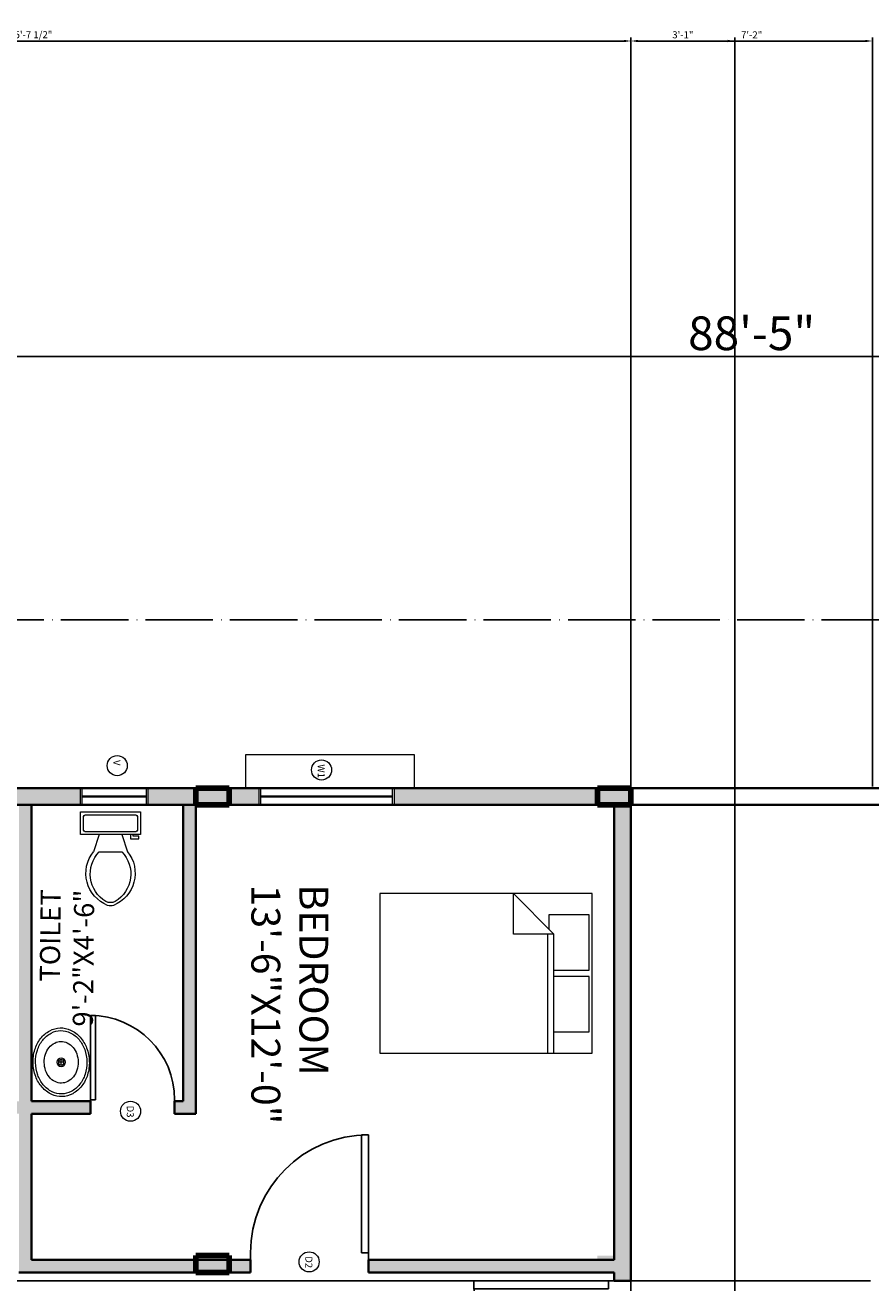
# Model space of a CAD drawing. Units: inches. Extents: x 7028582 to 7030319, y 63109697 to 63111305.
# Tile 12 of 18: x 7029446 to 7029748, y 63110857 to 63111305. Entities that reach past the tile are written whole.
import ezdxf

# ---------------------------------------------------------------- set-up
doc = ezdxf.new("R2010")
doc.units = ezdxf.units.IN
doc.linetypes.add('ACAD_ISO04W100', pattern=[30, 24, -3, 0, -3])
for name, color, linetype, lineweight in [('A-AREA-IDEN', 7, 'Continuous', 18), ('A-DOOR-IDEN', 20, 'Continuous', 13), ('A-FLOR-FIXT', 9, 'Continuous', 18), ('A-GLAZ-IDEN', 20, 'Continuous', 13), ('A-WALL-PATT', 8, 'Continuous', 13), ('C-ANNO-DIMS', 7, 'Continuous', 18), ('C-PROP', 1, 'ACAD_ISO04W100', 25), ('doors', 20, 'Continuous', 25), ('furniture', 9, 'Continuous', 18), ('PILLARS', 220, 'Continuous', 100), ('S-COLS-PATT', 220, 'Continuous', 100), ('walls', 6, 'Continuous', 35), ('WINDOW SHADOW', 9, 'Continuous', 13), ('windows', 5, 'Continuous', 18)]:
    doc.layers.add(name, color=color, linetype=linetype, lineweight=lineweight)
doc.styles.get("Standard").update_dxf_attribs({"font": 'arial.ttf'})
doc.dimstyles.new('ISO-25', dxfattribs={"dimtxt": 2.5, "dimasz": 2.5, "dimexe": 1.25, "dimexo": 0.625, "dimtad": 1, "dimlunit": 4, "dimtxsty": 'Standard', "dimcen": 2.5, "dimadec": 0, "dimazin": 0, "dimtfac": 1, "dimtmove": 0, "dimatfit": 3, "dimfxl": 1, "dimarcsym": 0})

# ---------------------------------------------------------------- blocks, each defined once
blk = doc.blocks.new('*U2')
for p, q in [((0, 0), (0, -5)), ((30, 0), (30, -5))]:
    blk.add_line(p, q)
blk.add_lwpolyline([(0, 0), (0, 30), (1.75, 30), (1.75, 0)], close=True)
blk.add_arc((0, 0), 30, 0, 90)
blk = doc.blocks.new('Toilet - top')
for p, q in [((9.5, -6), (9.5, -2)), ((-10, -8.5), (-8, -8.5)), ((-10, -9.5), (-10, -8.5)), ((-8, -8.5), (-8, -8)), ((-7, -8), (-7, -9.5)), ((-4, -8), (-6, -14)), ((4, -8), (6, -14)), ((-7, -9.5), (-10, -9.5)), ((4, -14), (-4, -14))]:
    blk.add_line(p, q)
blk.add_lwpolyline([(10.5, -8), (10.5, 0), (-10.5, 0), (-10.5, -8)], close=True)
for points in [[(-9.5, -2), (-9.5, -6)], [(8.5, -1), (-8.5, -1)], [(-8.5, -7), (8.5, -7)]]:
    blk.add_lwpolyline(points)
for centre, radius, start, end in [((-8.62, -1.88), 0.884, 81.8699, 188.1301), ((8.62, -1.88), 0.884, 351.8699, 98.1301), ((-8.62, -6.12), 0.884, 171.8699, 278.1301), ((8.62, -6.12), 0.884, 261.8699, 8.1301), ((3.52, -21.58), 12.17, 141.4691, 247.9714), ((4.2, -21.82), 11.33, 136.3677, 238.9468), ((-3.52, -21.58), 12.17, 292.0284, 38.5307), ((-4.2, -21.82), 11.33, 301.053, 43.6321), ((0, -27.88), 4, 245.7318, 294.2682), ((0, -29), 4, 254.8605, 285.1395)]:
    blk.add_arc(centre, radius, start, end)
blk = doc.blocks.new('Sink - Oval top')
for p, q in [((-1, 0), (1, 0)), ((0, 1), (0, -1))]:
    blk.add_line(p, q)
for points in [[(-12.23, 0.39, 0.117634), (-11.46, -3.36, 0.104469), (-8.88, -6.8, 0.090016), (-5.08, -9.07, 0.08192), (-0.32, -10.02, 0.08192), (4.49, -9.38, 0.090016), (8.42, -7.36, 0.104469), (11.22, -4.09, 0.117634), (12.23, -0.39, 0.117634), (11.46, 3.36, 0.104469), (8.88, 6.8, 0.090016), (5.08, 9.07, 0.08192), (0.32, 10.02, 0.08192), (-4.49, 9.38, 0.090016), (-8.42, 7.36, 0.104469), (-11.22, 4.09, 0.117634)], [(-11.29, 0.16, 0.118622), (-10.52, -3.25, 0.104678), (-8.07, -6.36, 0.089562), (-4.54, -8.37, 0.081185), (-0.13, -9.15, 0.081185), (4.3, -8.49, 0.089562), (7.89, -6.58, 0.104678), (10.42, -3.55, 0.118622), (11.29, -0.16, 0.118622), (10.52, 3.25, 0.104678), (8.07, 6.36, 0.089562), (4.54, 8.37, 0.081185), (0.13, 9.15, 0.081185), (-4.3, 8.49, 0.089562), (-7.89, 6.58, 0.104678), (-10.42, 3.55, 0.118622)], [(-7.42, 0.08, 0.118283), (-6.91, -2.17, 0.104607), (-5.29, -4.21, 0.089718), (-2.97, -5.53, 0.081436), (-0.07, -6.04, 0.081436), (2.84, -5.59, 0.089718), (5.2, -4.33, 0.104607), (6.86, -2.32, 0.118283), (7.42, -0.08, 0.118283), (6.91, 2.17, 0.104607), (5.29, 4.21, 0.089718), (2.97, 5.53, 0.081436), (0.07, 6.04, 0.081436), (-2.84, 5.59, 0.089718), (-5.2, 4.33, 0.104607), (-6.86, 2.32, 0.118283)]]:
    blk.add_lwpolyline(points, format="xyb", close=True)
for radius in [1.5, 1]:
    blk.add_circle((0, 0), radius)
blk = doc.blocks.new('Bed - Queen')
for p, q in [((0, -80.00003), (0, 0)), ((0, 0), (59.99999, 0)), ((59.99999, 0), (59.99999, -80.00003)), ((7.99999, -1.2), (28.79998, -1.2)), ((7.99999, -14.4), (7.99999, -1.2)), ((28.79998, -1.2), (28.79998, -14.4)), ((31.19999, -1.2), (51.99999, -1.2)), ((31.19999, -14.4), (31.19999, -1.2)), ((51.99999, -1.2), (51.99999, -16.4)), ((0, -14.4), (44.8, -14.4)), ((44.8, -16.8), (0, -16.8)), ((59.99999, -29.6), (44.8, -14.4)), ((44.8, -14.4), (44.8, -29.6)), ((51.99999, -16.4), (46.79936, -16.4)), ((44.8, -29.6), (59.99999, -29.6)), ((59.99999, -80.00003), (0, -80.00003))]:
    blk.add_line(p, q)
blk = doc.blocks.new('*D11')
at = {"layer": 'C-ANNO-DIMS', "color": 0, "lineweight": -2, "transparency": 16777216}
for p, q in [((7029174.71, 63111093.68), (7029174.71, 63111188.03)), ((7030233.21, 63111186.78), (7029177.21, 63111186.78)), ((7030235.71, 63111093.68), (7030235.71, 63111188.03))]:
    blk.add_line(p, q, dxfattribs=at)
at = {"layer": 'C-ANNO-DIMS', "color": 0, "lineweight": 100, "transparency": 16777216}
for points in [[(7029177.21, 63111187.2), (7029177.21, 63111186.36), (7029174.71, 63111186.78)], [(7030233.21, 63111187.2), (7030233.21, 63111186.36), (7030235.71, 63111186.78)]]:
    blk.add_solid(points, dxfattribs=at)
at = {"layer": 'Defpoints', "color": 0, "lineweight": 100, "transparency": 16777216}
for p in [(7029174.71, 63111186.78), (7029174.71, 63111093.06), (7030235.71, 63111093.06)]:
    blk.add_point(p, dxfattribs=at)
at = {"layer": 'C-ANNO-DIMS', "color": 0, "transparency": 16777216, "insert": (7029705.21, 63111193.53), "char_height": 12, "attachment_point": 5}
blk.add_mtext('88\'-5"', dxfattribs=at)
blk = doc.blocks.new('WIN-SASH-24')
for p, q in [((24.05, 6), (0, 6)), ((0.5, 6), (0.5, 0)), ((23.55, 0), (23.55, 6)), ((0, 0), (24.05, 0)), ((23.55, 3.2), (0.5, 3.2)), ((23.55, 2.8), (0.5, 2.8))]:
    blk.add_line(p, q)
blk = doc.blocks.new('WIN-SASH-48')
for p, q in [((48.05, 6), (0, 6)), ((0.5, 6), (0.5, 0)), ((47.55, 0), (47.55, 6)), ((47.55, 3.2), (0.5, 3.2)), ((47.55, 2.8), (0.5, 2.8)), ((0, 0), (48.05, 0))]:
    blk.add_line(p, q)
blk = doc.blocks.new('WINDOW-SHADE-HEAD-60')
for p, q in [((60.25, 11.9), (0, 11.9)), ((0, 11.9), (0, 0)), ((60.25, 0), (60.25, 11.9))]:
    blk.add_line(p, q)
blk = doc.blocks.new('COLUMN-RECT-PROFILE')
for p, q in [((11.91, 6), (0, 6)), ((0, 6), (0, 0)), ((11.91, 0), (11.91, 6)), ((0, 0), (11.91, 0))]:
    blk.add_line(p, q)
blk = doc.blocks.new('TAG-D2-MT-L')
blk.add_circle((3.58, 3.58), 3.58)
at = {"insert": (2.23, 5.6), "char_height": 2.5, "attachment_point": 7, "rotation": 270}
blk.add_mtext_dynamic_manual_height_columns('D2', width=2.5021, gutter_width=12.5, heights=[0], dxfattribs=at)
blk = doc.blocks.new('TAG-D3-MT-L')
blk.add_circle((3.58, 3.58), 3.58)
at = {"insert": (2.23, 5.6), "char_height": 2.5, "attachment_point": 7, "rotation": 270}
blk.add_mtext_dynamic_manual_height_columns('D3', width=2.5021, gutter_width=12.5, heights=[0], dxfattribs=at)
blk = doc.blocks.new('TAG-V-MT-L')
blk.add_circle((3.58, 3.58), 3.58)
at = {"insert": (2.23, 5.6), "char_height": 2.5, "attachment_point": 7, "rotation": 270}
blk.add_mtext_dynamic_manual_height_columns('V', width=2.5021, gutter_width=12.5, heights=[0], dxfattribs=at)
blk = doc.blocks.new('TAG-W1-MT-L')
blk.add_circle((3.58, 3.58), 3.58)
at = {"insert": (2.23, 5.6), "char_height": 2.5, "attachment_point": 7, "rotation": 270}
blk.add_mtext_dynamic_manual_height_columns('W1', width=2.5021, gutter_width=12.5, heights=[0], dxfattribs=at)
blk = doc.blocks.new('*D102')
at = {"layer": 'C-ANNO-DIMS', "color": 0, "lineweight": -2, "transparency": 16777216}
for p, q in [((7029662.21, 63111033.68), (7029662.21, 63111300.44)), ((7029664.71, 63111299.19), (7029745.71, 63111299.19)), ((7029748.21, 63111033.68), (7029748.21, 63111300.44))]:
    blk.add_line(p, q, dxfattribs=at)
at = {"layer": 'C-ANNO-DIMS', "color": 0, "lineweight": 100, "transparency": 16777216}
for points in [[(7029664.71, 63111299.61), (7029664.71, 63111298.77), (7029662.21, 63111299.19)], [(7029745.71, 63111299.61), (7029745.71, 63111298.77), (7029748.21, 63111299.19)]]:
    blk.add_solid(points, dxfattribs=at)
at = {"layer": 'Defpoints', "color": 0, "lineweight": 100, "transparency": 16777216}
for p in [(7029748.21, 63111299.19), (7029662.21, 63111033.06), (7029748.21, 63111033.06)]:
    blk.add_point(p, dxfattribs=at)
at = {"layer": 'C-ANNO-DIMS', "color": 0, "transparency": 16777216, "insert": (7029705.21, 63111301.07), "char_height": 2.5, "attachment_point": 5}
blk.add_mtext('7\'-2"', dxfattribs=at)
blk = doc.blocks.new('*D104')
at = {"layer": 'C-ANNO-DIMS', "color": 0, "lineweight": -2, "transparency": 16777216}
for p, q in [((7029747.58, 63110857.56), (7028586.23, 63110857.56)), ((7028587.48, 63110812.06), (7028587.48, 63110855.06)), ((7029747.58, 63110809.56), (7028586.23, 63110809.56))]:
    blk.add_line(p, q, dxfattribs=at)
at = {"layer": 'C-ANNO-DIMS', "color": 0, "lineweight": 100, "transparency": 16777216}
for points in [[(7028587.06, 63110855.06), (7028587.89, 63110855.06), (7028587.48, 63110857.56)], [(7028587.06, 63110812.06), (7028587.89, 63110812.06), (7028587.48, 63110809.56)]]:
    blk.add_solid(points, dxfattribs=at)
at = {"layer": 'Defpoints', "color": 0, "lineweight": 100, "transparency": 16777216}
for p in [(7028587.48, 63110857.56), (7029748.21, 63110857.56), (7029748.21, 63110809.56)]:
    blk.add_point(p, dxfattribs=at)
at = {"layer": 'C-ANNO-DIMS', "color": 0, "transparency": 16777216, "insert": (7028585.57, 63110833.56), "char_height": 2.5, "attachment_point": 5, "rotation": 90}
blk.add_mtext('4\'-0"', dxfattribs=at)
blk = doc.blocks.new('*D108')
at = {"layer": 'C-ANNO-DIMS', "color": 0, "lineweight": -2, "transparency": 16777216}
for p, q in [((7029662.21, 63110129.18), (7029662.21, 63111300.44)), ((7029664.71, 63111299.19), (7029696.71, 63111299.19)), ((7029699.21, 63110129.18), (7029699.21, 63111300.44))]:
    blk.add_line(p, q, dxfattribs=at)
at = {"layer": 'C-ANNO-DIMS', "color": 0, "lineweight": 100, "transparency": 16777216}
for points in [[(7029664.71, 63111299.61), (7029664.71, 63111298.77), (7029662.21, 63111299.19)], [(7029696.71, 63111299.61), (7029696.71, 63111298.77), (7029699.21, 63111299.19)]]:
    blk.add_solid(points, dxfattribs=at)
at = {"layer": 'Defpoints', "color": 0, "lineweight": 100, "transparency": 16777216}
for p in [(7029699.21, 63111299.19), (7029662.21, 63110128.56), (7029699.21, 63110128.56)]:
    blk.add_point(p, dxfattribs=at)
at = {"layer": 'C-ANNO-DIMS', "color": 0, "transparency": 16777216, "insert": (7029680.71, 63111301.09), "char_height": 2.5, "attachment_point": 5}
blk.add_mtext('3\'-1"', dxfattribs=at)
blk = doc.blocks.new('*D111')
at = {"layer": 'C-ANNO-DIMS', "color": 0, "lineweight": -2, "transparency": 16777216}
for p, q in [((7029234.71, 63111033.68), (7029234.71, 63111300.44)), ((7029237.21, 63111299.19), (7029659.71, 63111299.19)), ((7029662.21, 63111033.68), (7029662.21, 63111300.44))]:
    blk.add_line(p, q, dxfattribs=at)
at = {"layer": 'C-ANNO-DIMS', "color": 0, "lineweight": 100, "transparency": 16777216}
for points in [[(7029237.21, 63111299.61), (7029237.21, 63111298.77), (7029234.71, 63111299.19)], [(7029659.71, 63111299.61), (7029659.71, 63111298.77), (7029662.21, 63111299.19)]]:
    blk.add_solid(points, dxfattribs=at)
at = {"layer": 'Defpoints', "color": 0, "lineweight": 100, "transparency": 16777216}
for p in [(7029662.21, 63111299.19), (7029234.71, 63111033.06), (7029662.21, 63111033.06)]:
    blk.add_point(p, dxfattribs=at)
at = {"layer": 'C-ANNO-DIMS', "color": 0, "transparency": 16777216, "insert": (7029448.46, 63111301.11), "char_height": 2.5, "attachment_point": 5}
blk.add_mtext('35\'-7 1/2"', dxfattribs=at)
blk = doc.blocks.new('*D112')
at = {"layer": 'C-ANNO-DIMS', "color": 0, "lineweight": -2, "transparency": 16777216}
for p, q in [((7029747.58, 63111033.06), (7028586.23, 63111033.06)), ((7028587.48, 63111030.56), (7028587.48, 63110548.06)), ((7029747.58, 63110545.56), (7028586.23, 63110545.56))]:
    blk.add_line(p, q, dxfattribs=at)
at = {"layer": 'C-ANNO-DIMS', "color": 0, "lineweight": 100, "transparency": 16777216}
for points in [[(7028587.06, 63111030.56), (7028587.89, 63111030.56), (7028587.48, 63111033.06)], [(7028587.06, 63110548.06), (7028587.89, 63110548.06), (7028587.48, 63110545.56)]]:
    blk.add_solid(points, dxfattribs=at)
at = {"layer": 'Defpoints', "color": 0, "lineweight": 100, "transparency": 16777216}
for p in [(7029748.21, 63111033.06), (7028587.48, 63110545.56), (7029748.21, 63110545.56)]:
    blk.add_point(p, dxfattribs=at)
at = {"layer": 'C-ANNO-DIMS', "color": 0, "transparency": 16777216, "insert": (7028585.56, 63110789.31), "char_height": 2.5, "attachment_point": 5, "rotation": 90}
blk.add_mtext('40\'-7 1/2"', dxfattribs=at)

msp = doc.modelspace()

# ---------------------------------------------------------------- hatches: boundary and pattern name
at = {"layer": 'A-WALL-PATT'}
h = msp.add_hatch(color=256, dxfattribs=at)
h.dxf.hatch_style = 1
h.paths.add_polyline_path([(7029429.881, 63111027.057), (7029466.152, 63111027.057), (7029466.152, 63111033.057), (7029429.881, 63111033.057)])
h = msp.add_hatch(color=256, dxfattribs=at)
h.dxf.hatch_style = 1
h.paths.add_polyline_path([(7029490.2, 63111027.057), (7029529.793, 63111027.057), (7029529.793, 63111033.057), (7029490.2, 63111033.057)])
h = msp.add_hatch(color=256, dxfattribs=at)
h.dxf.hatch_style = 1
h.paths.add_polyline_path([(7029662.205, 63111033.057), (7029577.841, 63111033.057), (7029577.841, 63111027.057), (7029662.205, 63111027.057)])
h = msp.add_hatch(color=256, dxfattribs=at)
h.dxf.hatch_style = 1
h.paths.add_polyline_path([(7029384.705, 63111027.057), (7029389.205, 63111027.057), (7029389.205, 63110954.557), (7029384.705, 63110954.557)], flags=0)
h.paths.add_polyline_path([(7029384.705, 63110924.557), (7029389.205, 63110924.557), (7029389.205, 63110921.557), (7029444.205, 63110921.557), (7029444.205, 63111027.057), (7029448.705, 63111027.057), (7029448.705, 63110921.557), (7029469.705, 63110921.557), (7029469.705, 63110917.057), (7029448.705, 63110917.057), (7029448.705, 63110865.057), (7029526.726, 63110865.057), (7029526.726, 63110860.557), (7029444.205, 63110860.557), (7029444.205, 63110917.057), (7029389.205, 63110917.057), (7029389.205, 63110910.057), (7029384.705, 63110910.057)])
h = msp.add_hatch(color=256, dxfattribs=at)
h.dxf.hatch_style = 1
h.paths.add_polyline_path([(7029502.705, 63111027.057), (7029507.205, 63111027.057), (7029507.205, 63110917.057), (7029499.705, 63110917.057), (7029499.705, 63110921.557), (7029502.705, 63110921.557)], flags=17)
h = msp.add_hatch(color=256, dxfattribs=at)
h.dxf.hatch_style = 1
h.paths.add_polyline_path([(7029662.205, 63111027.057), (7029656.205, 63111027.057), (7029656.205, 63110865.057), (7029568.726, 63110865.057), (7029568.726, 63110860.557), (7029656.205, 63110860.557), (7029656.205, 63110857.557), (7029662.205, 63110857.557)])
at = {"layer": 'S-COLS-PATT'}
h = msp.add_hatch(color=256, dxfattribs=at)
h.dxf.hatch_style = 1
h.paths.add_polyline_path([(7029519.153, 63111033.057), (7029507.238, 63111033.057), (7029507.238, 63111027.057), (7029519.153, 63111027.057)])
h = msp.add_hatch(color=256, dxfattribs=at)
h.dxf.hatch_style = 1
h.paths.add_polyline_path([(7029519.153, 63111033.057), (7029507.238, 63111033.057), (7029507.238, 63111027.057), (7029519.153, 63111027.057)])
h = msp.add_hatch(color=256, dxfattribs=at)
h.dxf.hatch_style = 1
h.paths.add_polyline_path([(7029662.205, 63111033.057), (7029650.291, 63111033.057), (7029650.291, 63111027.057), (7029662.205, 63111027.057)])
h = msp.add_hatch(color=256, dxfattribs=at)
h.dxf.hatch_style = 1
h.paths.add_polyline_path([(7029662.205, 63111033.057), (7029650.291, 63111033.057), (7029650.291, 63111027.057), (7029662.205, 63111027.057)])
h = msp.add_hatch(color=256, dxfattribs=at)
h.dxf.hatch_style = 1
h.paths.add_polyline_path([(7029662.205, 63111033.057), (7029650.291, 63111033.057), (7029650.291, 63111027.057), (7029662.205, 63111027.057)])
h = msp.add_hatch(color=256, dxfattribs=at)
h.dxf.hatch_style = 1
h.paths.add_polyline_path([(7029662.205, 63110866.557), (7029650.291, 63110866.557), (7029650.291, 63110860.557), (7029662.205, 63110860.557)])

# ---------------------------------------------------------------- linework, layer by layer
at = {"layer": 'C-PROP'}
msp.add_line((7030235.705, 63111093.057), (7029174.705, 63111093.057), dxfattribs=at)
at = {"layer": 'PILLARS'}
for p, q in [((7029519.153, 63111033.057), (7029507.238, 63111033.057)), ((7029507.238, 63111033.057), (7029507.238, 63111027.057)), ((7029519.153, 63111027.057), (7029519.153, 63111033.057)), ((7029662.205, 63111033.057), (7029650.291, 63111033.057)), ((7029650.291, 63111033.057), (7029650.291, 63111027.057)), ((7029662.205, 63111027.057), (7029662.205, 63111033.057)), ((7029507.238, 63111027.057), (7029519.153, 63111027.057)), ((7029650.291, 63111027.057), (7029662.205, 63111027.057))]:
    msp.add_line(p, q, dxfattribs=at)
at = {"layer": 'walls'}
for p, q in [((7030175.705, 63111033.057), (7029234.705, 63111033.057)), ((7029234.705, 63111033.057), (7030175.705, 63111033.057)), ((7029662.205, 63110857.557), (7029662.205, 63111033.057)), ((7030169.705, 63111027.057), (7029240.705, 63111027.057)), ((7029240.705, 63111027.057), (7030169.705, 63111027.057)), ((7029448.705, 63110921.557), (7029448.705, 63111027.057)), ((7029502.705, 63110921.557), (7029502.705, 63111027.057)), ((7029507.205, 63110917.057), (7029507.205, 63111027.057)), ((7029656.205, 63110865.057), (7029656.205, 63111027.057)), ((7029448.705, 63110921.557), (7029469.705, 63110921.557)), ((7029469.705, 63110917.057), (7029469.705, 63110921.557)), ((7029499.705, 63110921.557), (7029502.705, 63110921.557)), ((7029502.705, 63110921.557), (7029499.705, 63110921.557)), ((7029499.705, 63110921.557), (7029499.705, 63110917.057)), ((7029448.705, 63110865.057), (7029448.705, 63110917.057)), ((7029448.705, 63110917.057), (7029469.705, 63110917.057)), ((7029499.705, 63110917.057), (7029507.205, 63110917.057)), ((7029448.705, 63110865.057), (7029526.726, 63110865.057)), ((7029526.726, 63110860.557), (7029526.726, 63110865.057)), ((7029568.726, 63110865.057), (7029656.205, 63110865.057)), ((7029568.726, 63110865.057), (7029568.726, 63110860.557)), ((7029444.205, 63110860.557), (7029526.726, 63110860.557)), ((7029568.726, 63110860.557), (7029656.205, 63110860.557)), ((7029656.205, 63110857.557), (7029656.205, 63110860.557)), ((7029656.205, 63110860.557), (7029656.205, 63110857.557)), ((7029656.205, 63110857.557), (7029662.205, 63110857.557))]:
    msp.add_line(p, q, dxfattribs=at)
at = {"layer": 'windows'}
for p, q in [((7029466.152, 63111027.057), (7029466.152, 63111033.057)), ((7029490.2, 63111033.057), (7029490.2, 63111027.057)), ((7029529.793, 63111027.057), (7029529.793, 63111033.057)), ((7029577.841, 63111033.057), (7029577.841, 63111027.057))]:
    msp.add_line(p, q, dxfattribs=at)

# ---------------------------------------------------------------- block references
at = {"layer": 'A-DOOR-IDEN'}
for name, p in [('TAG-D3-MT-L', (7029480.418, 63110914.381)), ('TAG-D2-MT-L', (7029544.022, 63110860.722))]:
    msp.add_blockref(name, p, dxfattribs=at)
at = {"layer": 'A-FLOR-FIXT', "xscale": -1.013555723357934, "yscale": 1.013555723357934, "zscale": 1.013555723357934}
msp.add_blockref('Toilet - top', (7029476.859, 63111024.605), dxfattribs=at)
at = {"layer": 'A-FLOR-FIXT', "xscale": -1, "rotation": 270}
msp.add_blockref('Sink - Oval top', (7029459.289, 63110935.416), dxfattribs=at)
at = {"layer": 'A-GLAZ-IDEN'}
for name, p in [('TAG-V-MT-L', (7029475.673, 63111037.489)), ('TAG-W1-MT-L', (7029548.45, 63111035.953))]:
    msp.add_blockref(name, p, dxfattribs=at)
at = {"layer": 'doors'}
msp.add_blockref('*U2', (7029469.705, 63110922.057), dxfattribs=at)
at = {"layer": 'doors', "xscale": -1.399999999999999, "yscale": 1.399999999999999, "zscale": 1.399999999999999}
msp.add_blockref('*U2', (7029568.726, 63110867.557), dxfattribs=at)
at = {"layer": 'doors', "xscale": -1.599999999999999, "yscale": 1.599999999999999, "zscale": 1.599999999999999, "rotation": 90}
msp.add_blockref('*U2', (7029654.205, 63110857.557), dxfattribs=at)
at = {"layer": 'furniture', "xscale": -0.9464141645025947, "yscale": 0.9464141645025947, "zscale": 0.9464141645025947, "rotation": 270}
msp.add_blockref('Bed - Queen', (7029648.437, 63110938.688), dxfattribs=at)
at = {"layer": 'PILLARS'}
msp.add_blockref('COLUMN-RECT-PROFILE', (7029507.238, 63110860.557), dxfattribs=at)
at = {"layer": 'WINDOW SHADOW'}
msp.add_blockref('WINDOW-SHADE-HEAD-60', (7029524.913, 63111033.057), dxfattribs=at)
at = {"layer": 'windows'}
for name, p in [('WIN-SASH-24', (7029466.152, 63111027.057)), ('WIN-SASH-48', (7029529.793, 63111027.057))]:
    msp.add_blockref(name, p, dxfattribs=at)

# ---------------------------------------------------------------- texts
at = {"layer": 'A-AREA-IDEN'}
for s, width, gutter_width, insert, char_height, attachment_point, rotation in [('TOILET\\P9\'-2"X4\'-6"', 42.97461, 35.821, (7029452.002, 63110997.065), 7.16426, 3, 89.3536), ('BEDROOM\\P13\'-6"X12\'-0"', 82.04322, 51.315, (7029527.033, 63110998.737), 10.26307, 7, 270)]:
    msp.add_mtext_dynamic_manual_height_columns(s, width=width, gutter_width=gutter_width, heights=[0], dxfattribs=dict(at, insert=insert, char_height=char_height, attachment_point=attachment_point, rotation=rotation))

# ---------------------------------------------------------------- dimensions: what is measured, and where the dimension line sits
at = {"layer": 'C-ANNO-DIMS'}
for base, p1, p2, override, picture, middle in [((7029662.205, 63111299.19), (7029234.705, 63111033.057), (7029662.205, 63111033.057), {"dimdec": 1, "dimlfac": 1, "dimrnd": 0, "dimzin": 1, "dimdsep": 46, "dimlunit": 4, "dimfrac": 2}, '*D111', (7029448.455, 63111301.108)), ((7029699.205, 63111299.19), (7029662.205, 63110128.557), (7029699.205, 63110128.557), {"dimdec": 1, "dimlfac": 1, "dimrnd": 0, "dimzin": 1, "dimdsep": 46, "dimlunit": 4, "dimfrac": 2}, '*D108', (7029680.705, 63111301.092)), ((7029748.205, 63111299.19), (7029662.205, 63111033.057), (7029748.205, 63111033.057), {"dimdec": 1, "dimlfac": 1, "dimrnd": 0, "dimzin": 1, "dimdsep": 46, "dimlunit": 4, "dimfrac": 2}, '*D102', (7029705.205, 63111301.07)), ((7029174.705, 63111186.781), (7030235.705, 63111093.057), (7029174.705, 63111093.057), {"dimtxt": 12, "dimclrd": 0, "dimclre": 0, "dimclrt": 0}, '*D11', (7029705.205, 63111193.533))]:
    dim = msp.add_linear_dim(base=base, p1=p1, p2=p2, dimstyle='ISO-25', override=override, dxfattribs=at)
    dim.commit()
    dim.dimension.update_dxf_attribs({"geometry": picture, "text_midpoint": middle})
for base, p1, p2, picture, middle in [((7028587.475, 63110545.557), (7029748.205, 63111033.057), (7029748.205, 63110545.557), '*D112', (7028585.558, 63110789.307)), ((7028587.475, 63110857.557), (7029748.205, 63110809.557), (7029748.205, 63110857.557), '*D104', (7028585.574, 63110833.557))]:
    dim = msp.add_linear_dim(base=base, p1=p1, p2=p2, angle=90, dimstyle='ISO-25', override={"dimdec": 1, "dimlfac": 1, "dimrnd": 0, "dimzin": 1, "dimdsep": 46, "dimlunit": 4, "dimfrac": 2}, dxfattribs=at)
    dim.commit()
    dim.dimension.update_dxf_attribs({"geometry": picture, "text_midpoint": middle})

doc.saveas('drawing.dxf')
